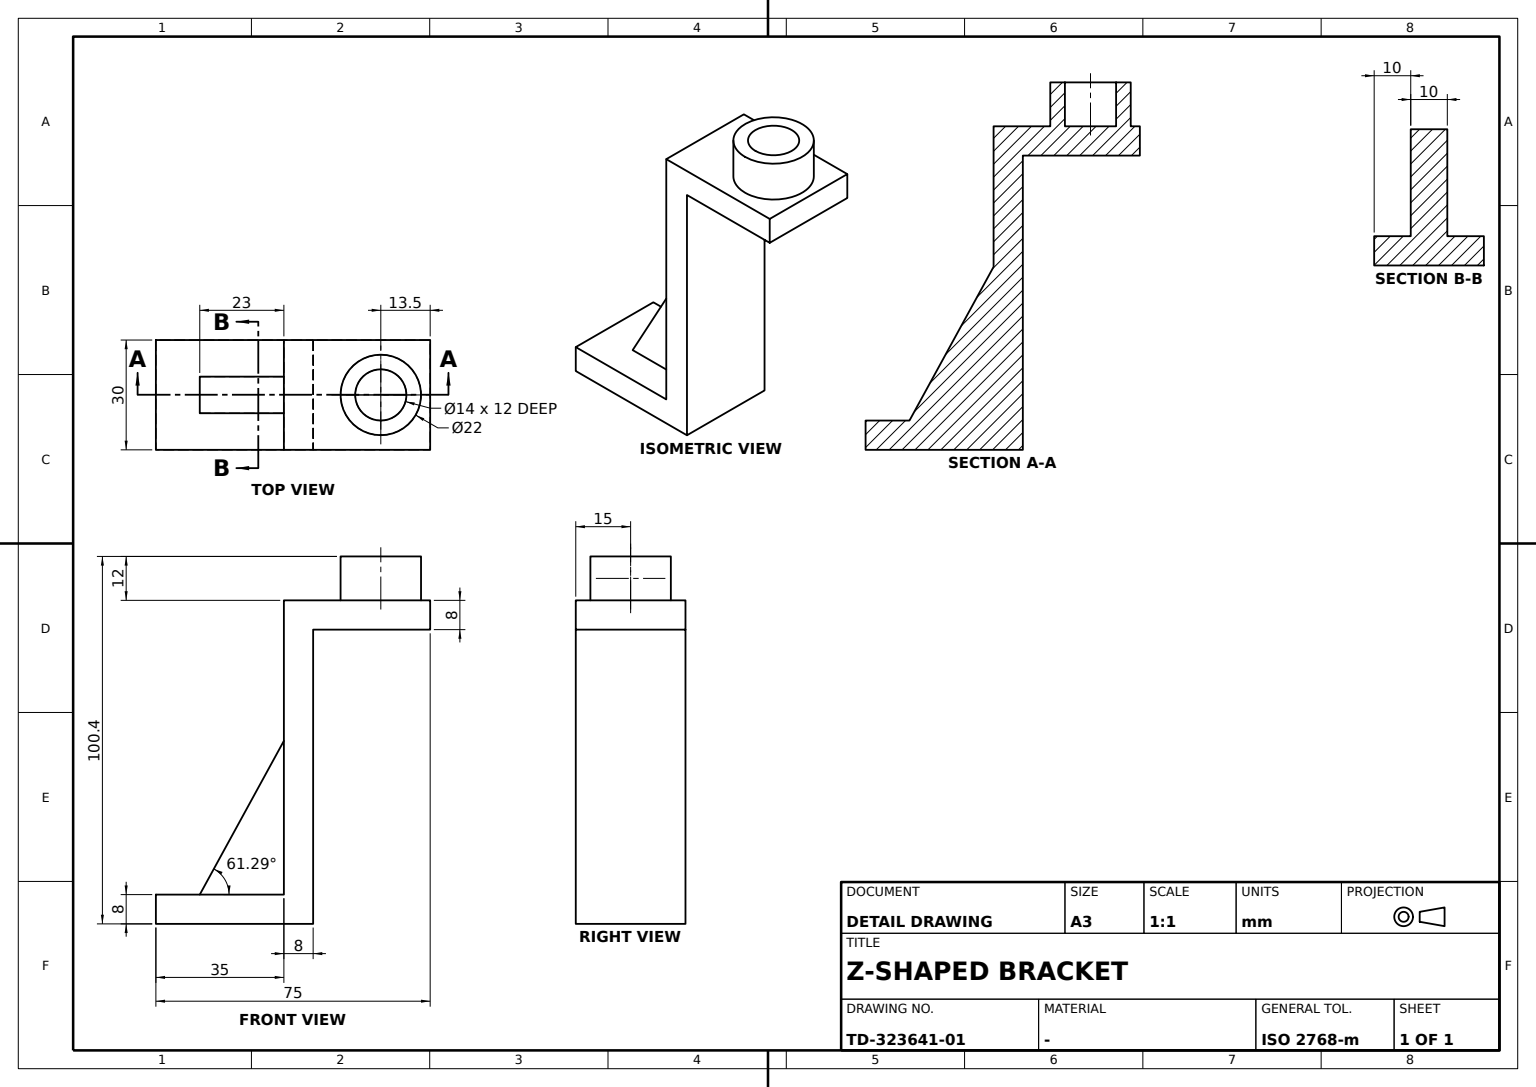
CATIA V5 part; units mm, degrees
sketch "Sketch1" plane through (0, 0, 0) normal (1, 0, 0) x (0, 1, 0)
  point P0 (-36.5013, -36.1992)
  line L0 (-36.5013, -36.1992) -> (-1.5013, -36.1992)
  point P1 (-1.5013, -36.1992)
  line L1 (-1.5013, -36.1992) -> (-1.5013, 44.1992)
  line L2 (-1.5013, 44.1992) -> (38.4987, 44.1992)
  line L3 (38.4987, 44.1992) -> (38.4987, 36.1992)
  point P2 (38.4987, 36.1992)
  line L4 (38.4987, 36.1992) -> (6.4987, 36.1992)
  line L5 (6.4987, 36.1992) -> (6.4987, -44.1992)
  line L6 (6.4987, -44.1992) -> (-36.5013, -44.1992)
  line L7 (-36.5013, -44.1992) -> (-36.5013, -36.1992)
  dimension "distance P0 P1" = 35
  dimension "distance P1 P2 x axis" = 40
  dimension "length L3" = 8
  dimension "length L7" = 8
  dimension "distance L1 L5" = 8
  constraint horizontal L0 x-axis
  constraint horizontal L2 x-axis
  constraint horizontal L4 x-axis
  constraint horizontal L6 x-axis
  constraint vertical L1 y-axis
  constraint vertical L3 y-axis
  constraint vertical L5 y-axis
  constraint vertical L7 y-axis
  constraint symmetry L2 L6 x-axis
extrude "Pad1" add sketch "Sketch1" along normal blind 30
sketch "Sketch2" plane through (0, 0, 44.1992) normal (0, 0, 1) x (1, 0, 0)
  circle A0 centre (15, 25) radius 7
  point P0 (15, 25)
  circle A1 centre (15, 25) radius 11
  dimension "radius A1" = 11
  dimension "radius A0" = 7
  dimension "distance x axis P0" = 25
  dimension "distance P0 y axis" = 15
extrude "Pad2" add sketch "Sketch2" along normal blind 12
ref_plane "Plane1" through (15, 0, 0) normal (1, 0, 0) x (0, 1, 0)
sketch "Sketch3" plane through (15, 0, 0) normal (1, 0, 0) x (0, 1, 0)
  line L0 (-24.5013, -36.1992) -> (-1.5013, -36.1992)
  line L1 (-1.5013, -36.1992) -> (-1.5013, 5.8008)
  line L2 (-1.5013, 5.8008) -> (-24.5013, -36.1992)
  line L3 (-1.5013, -36.1992) -> (-36.5013, -36.1992) construction
  line L4 (-1.5013, 44.1992) -> (-1.5013, -36.1992) construction
  dimension "length L0" = 23
  dimension "length L1" = 42
  constraint horizontal L0 x-axis
  constraint vertical L1 y-axis
  constraint coincidence L0 L3
  constraint coincidence L1 L4
extrude "Pad3" add sketch "Sketch3" along normal mid plane 10
sketch "Pocket1 profile" plane through (0, 0, 44.1992) normal (0, 0, 1) x (1, 0, 0)
  circle A0 centre (15, 25) radius 7
extrude "Pocket1" cut sketch "Pocket1 profile" along normal blind 5
